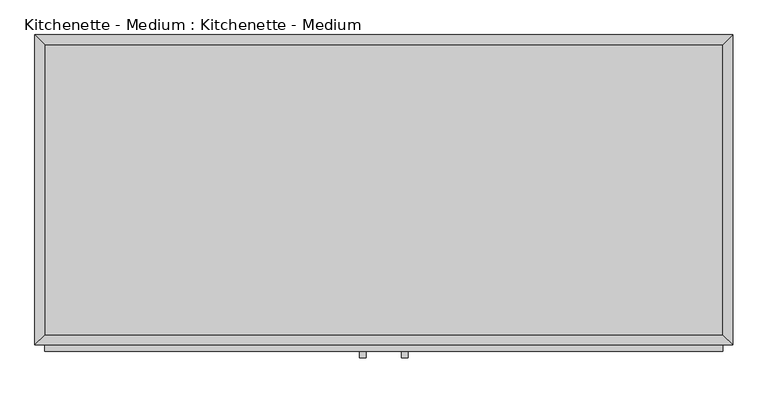
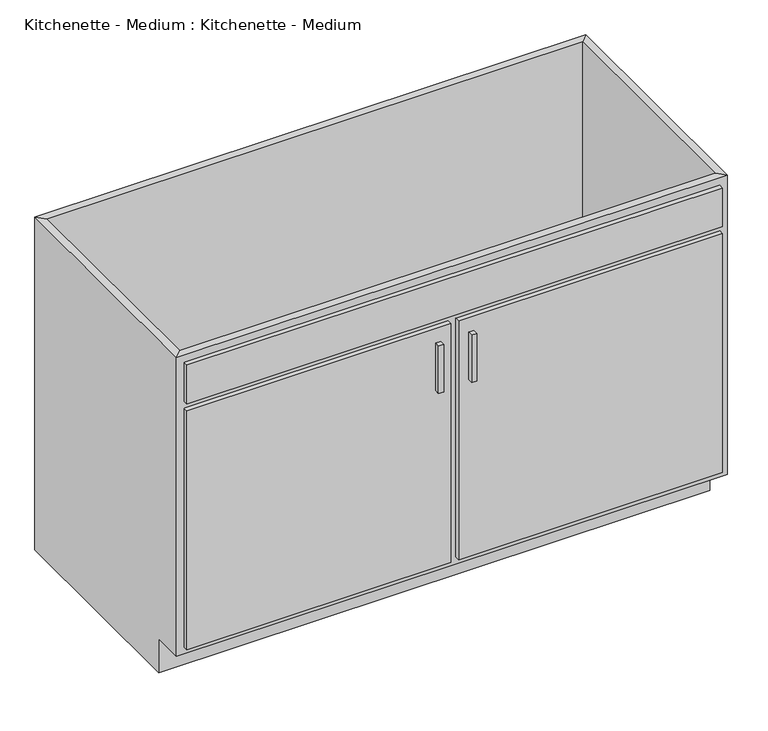
"""IFC4 building model written with IfcOpenShell, lengths in millimetres: proxy geometry, Kitchenette - Medium : Kitchenette - Medium."""

from ifc_helpers import new_model, si_unit, frame, origin, place, context, project, spatial, polyline, outline, extrude, faceted_brep, source, transform, mapped, element, save


def kitchenette_medium_kitchenette_medium_844211aa(model_context):
    return source(origin(), model_context, "Body", "SolidModel", [
        faceted_brep([(685.4877049, -590.55, 876.3), (685.4877049, -590.55, 88.9), (-648.0122951, -590.55, 88.9), (-648.0122951, -590.55, 876.3), (-667.0622951, -609.6, 876.3), (704.5377049, -609.6, 876.3), (-667.0622951, -609.6, 88.9), (704.5377049, -609.6, 88.9), (-648.0122951, -533.4, 88.9), (-648.0122951, -19.05, 88.9), (-648.0122951, -19.05, 876.3), (-667.0622951, 0.0, 876.3), (-667.0622951, 0.0, 0.0), (-667.0622951, -533.4, 0.0), (-667.0622951, -533.4, 88.9), (685.4877049, -19.05, 88.9), (685.4877049, -19.05, 876.3), (704.5377049, 0.0, 876.3), (704.5377049, 0.0, 0.0), (685.4877049, -533.4, 88.9), (704.5377049, -533.4, 88.9), (704.5377049, -533.4, 0.0)], [[[0, 1, 2, 3]], [[0, 3, 4, 5]], [[5, 4, 6, 7]], [[2, 1, 7, 6]], [[3, 2, 8, 9, 10]], [[4, 3, 10, 11]], [[6, 4, 11, 12, 13, 14]], [[2, 6, 14, 8]], [[10, 9, 15, 16]], [[11, 10, 16, 17]], [[12, 11, 17, 18]], [[1, 0, 16, 15, 19]], [[0, 5, 17, 16]], [[5, 7, 20, 21, 18, 17]], [[7, 1, 19, 20]], [[8, 19, 15, 9]], [[18, 21, 13, 12]], [[13, 21, 20, 19, 8, 14]]]),
        extrude(outline(polyline([(-16.1872951, -635.0), (-28.8872951, -635.0), (-28.8872951, -622.3), (-16.1872951, -622.3), (-16.1872951, -635.0)])), frame((0.0, 0.0, 573.769895), z_axis=(0.0, 0.0, 1.0), x_axis=(1.0, 0.0, 0.0)), (0.0, 0.0, 1.0), 124.730105),
        extrude(outline(polyline([(66.3627049, -635.0), (53.6627049, -635.0), (53.6627049, -622.3), (66.3627049, -622.3), (66.3627049, -635.0)])), frame((0.0, 0.0, 573.769895), z_axis=(0.0, 0.0, 1.0), x_axis=(1.0, 0.0, 0.0)), (0.0, 0.0, 1.0), 124.730105),
        extrude(outline(polyline([(685.4877049, -19.05), (685.4877049, -590.55), (-648.0122951, -590.55), (-648.0122951, -19.05), (685.4877049, -19.05)])), frame((0.0, 0.0, 88.9), z_axis=(0.0, 0.0, 1.0), x_axis=(1.0, 0.0, 0.0)), (0.0, 0.0, 1.0), 19.05),
        extrude(outline(polyline([(9.2127049, -622.3), (-648.0122951, -622.3), (-648.0122951, -609.6), (9.2127049, -609.6), (9.2127049, -622.3)])), frame((0.0, 0.0, 107.95), z_axis=(0.0, 0.0, 1.0), x_axis=(1.0, 0.0, 0.0)), (0.0, 0.0, 1.0), 628.65),
        extrude(outline(polyline([(685.4877049, -622.3), (28.2627049, -622.3), (28.2627049, -609.6), (685.4877049, -609.6), (685.4877049, -622.3)])), frame((0.0, 0.0, 107.95), z_axis=(0.0, 0.0, 1.0), x_axis=(1.0, 0.0, 0.0)), (0.0, 0.0, 1.0), 628.65),
        extrude(outline(polyline([(685.4877049, -622.3), (-648.0122951, -622.3), (-648.0122951, -609.6), (685.4877049, -609.6), (685.4877049, -622.3)])), frame((0.0, 0.0, 755.65), z_axis=(0.0, 0.0, 1.0), x_axis=(1.0, 0.0, 0.0)), (0.0, 0.0, 1.0), 101.6),
    ])


if __name__ == "__main__":
    model = new_model("IFC4")
    model_context = context("Model", 3, world=origin())
    ifc_project = project(units=[si_unit("LENGTHUNIT", "METRE", prefix="MILLI")], contexts=[model_context])
    site = spatial("IfcSite", under=ifc_project)
    building = spatial("IfcBuilding", under=site)
    placement = place(None, origin())
    kitchenette_medium_kitchenette_medium_shape = kitchenette_medium_kitchenette_medium_844211aa(model_context)
    element("IfcBuildingElementProxy", 1, Name="Kitchenette - Medium : Kitchenette - Medium", ObjectType="Kitchenette - Medium : Kitchenette - Medium", at=placement, inside=building, context=model_context, shape_type="MappedRepresentation", body=[
        mapped(kitchenette_medium_kitchenette_medium_shape, transform((0.0, 0.0, 0.0), x_axis=(1.0, 0.0, 0.0), y_axis=(0.0, 1.0, 0.0), z_axis=(0.0, 0.0, 1.0))),
    ])
    save(model, "model.ifc")

# Revit data of these elements
# Type "Kitchenette - Medium : Kitchenette - Medium"
#   Assembly Code = "E1090400"
#   Counter Length = 5' - 9"
#   Cabinet Width = 4' - 6"
#   Cabinet Height = 2' - 10 1/2"
#   Cabinet Depth = 2' - 0"
#   Toe Depth = 0' - 3"
#   Toe Height = 0' - 3 1/2"
#   Cabinet Material = Cabinets
#   Door/Drawer Material = Cabinets
#   Handle Material = Cabinets - Handles
#   Default Elevation = 0
# Element 1 (IfcBuildingElementProxy, "Kitchenette - Medium : Kitchenette - Medium")
#   Materials on its faces: "Cabinets", "Cabinets - Handles"
# Materials
#   "Cabinets": colour RGB 249 249 249, transparency 0
#   "Cabinets - Handles": class "Metal", colour RGB 57 57 57, transparency 0
